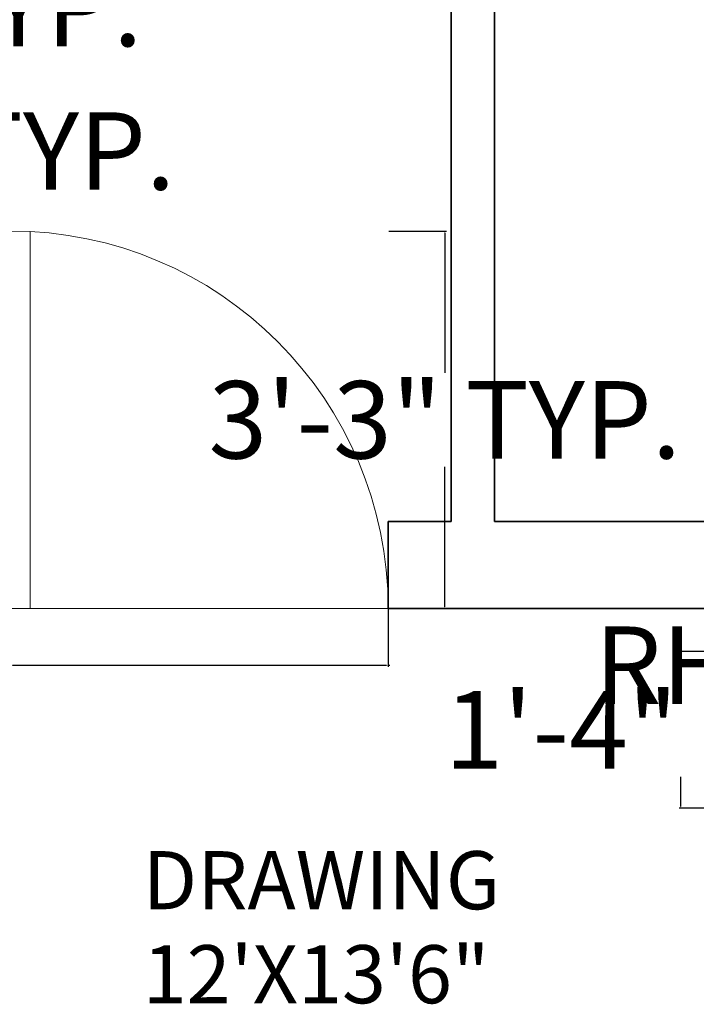
# Model space of a CAD drawing. Units: inches. Extents: x 125 to 976, y 231 to 853.
# Tile 5 of 16: x 324 to 393, y 453 to 555. Entities that reach past the tile are written whole.
import ezdxf

# ---------------------------------------------------------------- set-up
doc = ezdxf.new("R2010")
doc.units = ezdxf.units.IN
doc.header["$MEASUREMENT"] = 0
for name, color, linetype, lineweight in [('A-ANNO-DIMS', 2, 'Continuous', 18), ('A-AREA-IDEN', 7, 'Continuous', 18), ('A-DOOR', 3, 'Continuous', 18), ('A-WALL', 7, 'Continuous', 35)]:
    doc.layers.add(name, color=color, linetype=linetype, lineweight=lineweight)
doc.styles.get("Standard").update_dxf_attribs({"font": 'italic8.shx'})
doc.dimstyles.get("Standard").update_dxf_attribs({"dimtxt": 8, "dimasz": 0.18, "dimexe": 0.18, "dimexo": 0.0625, "dimgap": 0.09, "dimtad": 0, "dimtih": 1, "dimtoh": 1, "dimdec": 4, "dimzin": 0, "dimdsep": 46, "dimlunit": 3, "dimtxsty": 'Standard', "dimcen": 0.09, "dimclrt": 4, "dimadec": 0, "dimazin": 0, "dimtfac": 1, "dimtdec": 4, "dimtofl": 0, "dimtmove": 0, "dimatfit": 3, "dimfxl": 1, "dimtolj": 1, "dimtzin": 0, "dimarcsym": 0})

# ---------------------------------------------------------------- blocks, each defined once
blk = doc.blocks.new('DOOR-39IN-RH')
for p, q in [((0, 39), (0, 0)), ((2, 38.95), (2, 0)), ((0, 0), (39, 0))]:
    blk.add_line(p, q)
blk.add_arc((0, 0), 39, 0, 90)
blk = doc.blocks.new('*D40')
at = {"layer": 'A-ANNO-DIMS', "color": 0, "lineweight": -2, "transparency": 16777216}
for p, q in [((322.59, 494.04), (322.59, 488.07)), ((361.59, 494.04), (361.59, 488.07)), ((322.77, 488.25), (361.41, 488.25)), ((361.59, 488.25), (361.77, 488.25))]:
    blk.add_line(p, q, dxfattribs=at)
at = {"layer": 'A-ANNO-DIMS', "color": 0, "transparency": 16777216}
for points in [[(322.77, 488.28), (322.77, 488.22), (322.59, 488.25)], [(361.41, 488.28), (361.41, 488.22), (361.59, 488.25)]]:
    blk.add_solid(points, dxfattribs=at)
at = {"layer": 'Defpoints', "color": 0, "transparency": 16777216}
for p in [(322.59, 494.1), (361.59, 494.1), (361.59, 488.25)]:
    blk.add_point(p, dxfattribs=at)
at = {"layer": 'A-ANNO-DIMS', "color": 4, "transparency": 16777216, "insert": (432.52, 488.25), "char_height": 8, "attachment_point": 5}
blk.add_mtext('\\A1;RH DOOR 3\'-3" TYP.', dxfattribs=at)
blk = doc.blocks.new('*D41')
at = {"layer": 'A-ANNO-DIMS', "color": 0, "lineweight": -2, "transparency": 16777216}
for p, q in [((361.65, 533.1), (367.62, 533.1)), ((367.44, 532.92), (367.44, 518.46)), ((367.44, 494.28), (367.44, 508.75)), ((361.65, 494.1), (367.62, 494.1))]:
    blk.add_line(p, q, dxfattribs=at)
at = {"layer": 'A-ANNO-DIMS', "color": 0, "transparency": 16777216}
for points in [[(367.41, 532.92), (367.47, 532.92), (367.44, 533.1)], [(367.41, 494.28), (367.47, 494.28), (367.44, 494.1)]]:
    blk.add_solid(points, dxfattribs=at)
at = {"layer": 'Defpoints', "color": 0, "transparency": 16777216}
for p in [(361.59, 533.1), (367.44, 533.1), (361.59, 494.1)]:
    blk.add_point(p, dxfattribs=at)
at = {"layer": 'A-ANNO-DIMS', "color": 4, "transparency": 16777216, "insert": (367.44, 513.6), "char_height": 8, "attachment_point": 5}
blk.add_mtext('\\A1;3\'-3" TYP.', dxfattribs=at)
blk = doc.blocks.new('*D45')
at = {"layer": 'A-ANNO-DIMS', "color": 0, "lineweight": -2, "transparency": 16777216}
for p, q in [((394.8, 489.65), (391.65, 489.65)), ((391.83, 489.47), (391.83, 486.42)), ((391.83, 473.66), (391.83, 476.71)), ((394.8, 473.48), (391.65, 473.48))]:
    blk.add_line(p, q, dxfattribs=at)
at = {"layer": 'A-ANNO-DIMS', "color": 0, "transparency": 16777216}
for points in [[(391.8, 489.47), (391.86, 489.47), (391.83, 489.65)], [(391.8, 473.66), (391.86, 473.66), (391.83, 473.48)]]:
    blk.add_solid(points, dxfattribs=at)
at = {"layer": 'Defpoints', "color": 0, "transparency": 16777216}
for p in [(391.83, 489.65), (394.87, 489.65), (394.87, 473.48)]:
    blk.add_point(p, dxfattribs=at)
at = {"layer": 'A-ANNO-DIMS', "color": 4, "transparency": 16777216, "insert": (391.83, 481.57), "char_height": 8, "attachment_point": 5}
blk.add_mtext('\\A1;1\'-4" TYP.', dxfattribs=at)
blk = doc.blocks.new('*D46')
at = {"layer": 'A-ANNO-DIMS', "color": 0, "lineweight": -2, "transparency": 16777216}
for p, q in [((274.61, 567.59), (278.15, 567.59)), ((277.97, 567.41), (277.97, 561.05)), ((277.97, 544.97), (277.97, 551.34)), ((274.61, 544.79), (278.15, 544.79))]:
    blk.add_line(p, q, dxfattribs=at)
at = {"layer": 'A-ANNO-DIMS', "color": 0, "transparency": 16777216}
for points in [[(277.94, 567.41), (278, 567.41), (277.97, 567.59)], [(277.94, 544.97), (278, 544.97), (277.97, 544.79)]]:
    blk.add_solid(points, dxfattribs=at)
at = {"layer": 'Defpoints', "color": 0, "transparency": 16777216}
for p in [(274.55, 567.59), (277.97, 567.59), (274.55, 544.79)]:
    blk.add_point(p, dxfattribs=at)
at = {"layer": 'A-ANNO-DIMS', "color": 4, "transparency": 16777216, "insert": (277.97, 556.19), "char_height": 8, "attachment_point": 5}
blk.add_mtext('\\A1;DINING SET 1\'-11" TYP.', dxfattribs=at)
blk = doc.blocks.new('*D47')
at = {"layer": 'A-ANNO-DIMS', "color": 0, "lineweight": -2, "transparency": 16777216}
for p, q in [((252.38, 544.73), (252.38, 541.19)), ((274.55, 544.73), (274.55, 541.19)), ((252.56, 541.37), (274.37, 541.37)), ((274.55, 541.37), (274.73, 541.37))]:
    blk.add_line(p, q, dxfattribs=at)
at = {"layer": 'A-ANNO-DIMS', "color": 0, "transparency": 16777216}
for points in [[(252.56, 541.4), (252.56, 541.34), (252.38, 541.37)], [(274.37, 541.4), (274.37, 541.34), (274.55, 541.37)]]:
    blk.add_solid(points, dxfattribs=at)
at = {"layer": 'Defpoints', "color": 0, "transparency": 16777216}
for p in [(252.38, 544.79), (274.55, 544.79), (274.55, 541.37)]:
    blk.add_point(p, dxfattribs=at)
at = {"layer": 'A-ANNO-DIMS', "color": 4, "transparency": 16777216, "insert": (312.15, 541.37), "char_height": 8, "attachment_point": 5}
blk.add_mtext('\\A1;1\'-10" TYP.', dxfattribs=at)

msp = doc.modelspace()

# ---------------------------------------------------------------- linework, layer by layer
at = {"layer": 'A-WALL'}
for p, q in [((368.0792, 614.10475), (368.0792, 503.10475)), ((372.5792, 614.10475), (372.5792, 503.10475)), ((361.58656, 494.10475), (361.58656, 503.10475)), ((361.58656, 503.10475), (368.0792, 503.10475)), ((372.5792, 503.10475), (456.5792, 503.10475)), ((361.58656, 494.10475), (456.5792, 494.10475))]:
    msp.add_line(p, q, dxfattribs=at)

# ---------------------------------------------------------------- block references
at = {"layer": 'A-DOOR'}
msp.add_blockref('DOOR-39IN-RH', (322.58656, 494.10475), dxfattribs=at)

# ---------------------------------------------------------------- texts
at = {"layer": 'A-AREA-IDEN'}
for s, p in [('DRAWING', (336.22173, 463.0381)), ('12\'X13\'6"', (336.22173, 453.32381))]:
    msp.add_text(s, height=6, dxfattribs=at).set_placement(p)

# ---------------------------------------------------------------- dimensions: what is measured, and where the dimension line sits
at = {"layer": 'A-ANNO-DIMS'}
for base, p1, p2, text, picture, middle in [((277.96826, 567.59411), (274.54835, 544.79468), (274.54835, 567.59411), 'DINING SET <> TYP.', '*D46', (277.96826, 556.1944)), ((367.43656, 533.10475), (361.58656, 494.10475), (361.58656, 533.10475), '<> TYP.', '*D41', (367.43656, 513.60475)), ((391.83, 489.65243), (394.86616, 473.47878), (394.86616, 489.65243), '<> TYP.', '*D45', (391.83, 481.5656))]:
    dim = msp.add_linear_dim(base=base, p1=p1, p2=p2, angle=90, text=text, dimstyle='Standard', override={"dimdec": 1, "dimlfac": 1, "dimrnd": 0, "dimzin": 1, "dimdsep": 46, "dimlunit": 4, "dimfrac": 2}, dxfattribs=at)
    dim.commit()
    dim.dimension.update_dxf_attribs({"geometry": picture, "text_midpoint": middle})
for base, p1, p2, text, picture, middle in [((274.54835, 541.37477), (252.38252, 544.79468), (274.54835, 544.79468), '<> TYP.', '*D47', (312.15168, 541.37477)), ((361.58656, 488.25475), (322.58656, 494.10475), (361.58656, 494.10475), 'RH DOOR <> TYP.', '*D40', (432.52323, 488.25475))]:
    dim = msp.add_linear_dim(base=base, p1=p1, p2=p2, text=text, dimstyle='Standard', override={"dimdec": 1, "dimlfac": 1, "dimrnd": 0, "dimzin": 1, "dimdsep": 46, "dimlunit": 4, "dimfrac": 2}, dxfattribs=at)
    dim.commit()
    dim.dimension.update_dxf_attribs({"geometry": picture, "text_midpoint": middle})

doc.saveas('drawing.dxf')
